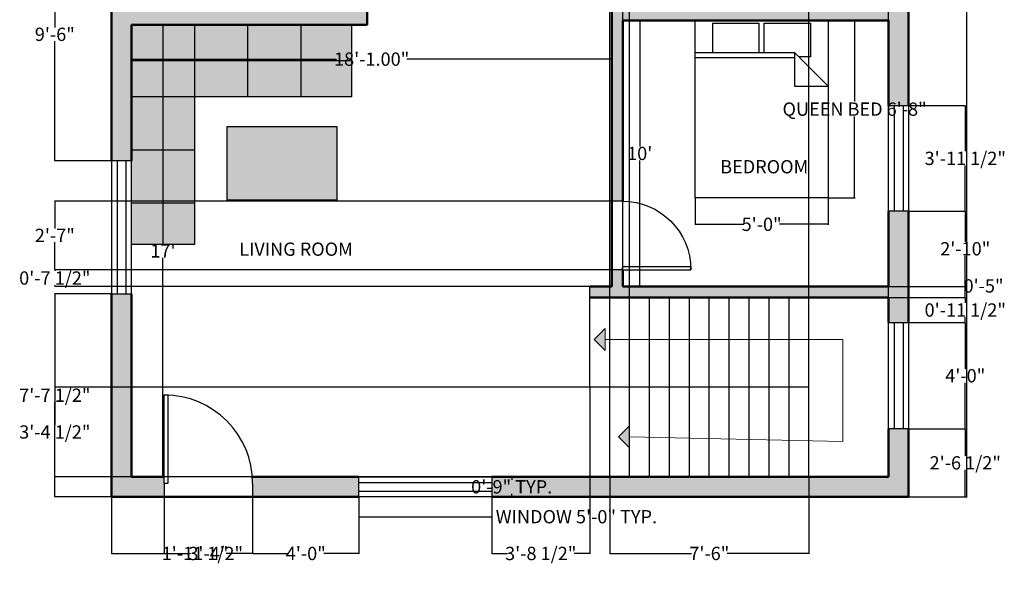
# Model space of a CAD drawing. Units: inches. Extents: x -19 to 426, y -15 to 535.
# Tile 1 of 4: x -19 to 426, y -15 to 235. Entities that reach past the tile are written whole.
import ezdxf

# ---------------------------------------------------------------- set-up
doc = ezdxf.new("R2010")
doc.units = ezdxf.units.IN
doc.header["$MEASUREMENT"] = 0
for name, color, linetype, lineweight in [('A-ANNO-DIMS', 3, 'Continuous', 18), ('A-ANNO-PATT', 18, 'Continuous', 13), ('A-ANNO-SYMB', 7, 'Continuous', 18), ('A-AREA-IDEN', 7, 'Continuous', 25), ('A-DOOR', 4, 'Continuous', 25), ('A-FLOR-STRS', 7, 'Continuous', 25), ('A-FURN', 40, 'Continuous', 25), ('A-FURN-PATT', 9, 'Continuous', 13), ('A-GLAZ', 40, 'Continuous', 25), ('A-WALL', 7, 'Continuous', 50), ('A-WALL-PATT', 5, 'Continuous', 13)]:
    doc.layers.add(name, color=color, linetype=linetype, lineweight=lineweight)
doc.styles.get("Standard").update_dxf_attribs({"font": 'arial.ttf'})
doc.dimstyles.get("Standard").update_dxf_attribs({"dimtxt": 6, "dimasz": 0.18, "dimexe": 0.18, "dimexo": 0.0625, "dimgap": 0.09, "dimtad": 0, "dimtih": 1, "dimtoh": 1, "dimzin": 0, "dimdsep": 46, "dimlunit": 3, "dimtxsty": 'Standard', "dimcen": 0.09, "dimadec": 0, "dimazin": 0, "dimtfac": 1, "dimtofl": 0, "dimtmove": 0, "dimatfit": 3, "dimfxl": 1, "dimtolj": 1, "dimtzin": 0, "dimarcsym": 0})

# ---------------------------------------------------------------- blocks, each defined once
blk = doc.blocks.new('*D1')
at = {"layer": 'A-ANNO-DIMS', "color": 0, "lineweight": -2, "transparency": 16777216}
for p, q in [((253.49, 235.01), (261.17, 235.01)), ((260.99, 234.83), (260.99, 178.16)), ((260.99, 115.19), (260.99, 171.85)), ((253.49, 115.01), (261.17, 115.01))]:
    blk.add_line(p, q, dxfattribs=at)
at = {"layer": 'A-ANNO-DIMS', "color": 0, "transparency": 16777216}
for points in [[(260.96, 234.83), (261.02, 234.83), (260.99, 235.01)], [(260.96, 115.19), (261.02, 115.19), (260.99, 115.01)]]:
    blk.add_solid(points, dxfattribs=at)
at = {"layer": 'Defpoints', "color": 0, "transparency": 16777216}
for p in [(253.43, 235.01), (260.99, 235.01), (253.43, 115.01)]:
    blk.add_point(p, dxfattribs=at)
at = {"layer": 'A-ANNO-DIMS', "color": 0, "transparency": 16777216, "insert": (260.99, 175.01), "char_height": 6, "attachment_point": 5}
blk.add_mtext("\\A1;10'", dxfattribs=at)
blk = doc.blocks.new('Bed - Queen')
for p, q in [((0, -80.00003), (0, 0)), ((0, 0), (59.99999, 0)), ((59.99999, 0), (59.99999, -80.00003)), ((7.99999, -1.2), (28.79998, -1.2)), ((7.99999, -14.4), (7.99999, -1.2)), ((28.79998, -1.2), (28.79998, -14.4)), ((31.19999, -1.2), (51.99999, -1.2)), ((31.19999, -14.4), (31.19999, -1.2)), ((51.99999, -1.2), (51.99999, -16.4)), ((0, -14.4), (44.8, -14.4)), ((44.8, -16.8), (0, -16.8)), ((59.99999, -29.6), (44.8, -14.4)), ((44.8, -14.4), (44.8, -29.6)), ((51.99999, -16.4), (46.79936, -16.4)), ((44.8, -29.6), (59.99999, -29.6)), ((59.99999, -80.00003), (0, -80.00003))]:
    blk.add_line(p, q)
blk = doc.blocks.new('*U9')
for p, q in [((0, 0), (0, -6)), ((40, 0), (40, -6))]:
    blk.add_line(p, q)
blk.add_lwpolyline([(0, 0), (0, 40), (1.75, 40), (1.75, 0)], close=True)
blk.add_arc((0, 0), 40, 0, 90)
blk = doc.blocks.new('*D16')
at = {"layer": 'A-ANNO-DIMS', "color": 0, "lineweight": -2, "transparency": 16777216}
for p, q in [((31.43, 232.94), (31.43, 217.39)), ((248.43, 232.94), (248.43, 217.39)), ((31.61, 217.57), (123.99, 217.57)), ((248.25, 217.57), (155.87, 217.57))]:
    blk.add_line(p, q, dxfattribs=at)
at = {"layer": 'A-ANNO-DIMS', "color": 0, "transparency": 16777216}
for points in [[(31.61, 217.6), (31.61, 217.54), (31.43, 217.57)], [(248.25, 217.6), (248.25, 217.54), (248.43, 217.57)]]:
    blk.add_solid(points, dxfattribs=at)
at = {"layer": 'Defpoints', "color": 0, "transparency": 16777216}
for p in [(31.43, 233.01), (248.43, 233.01), (248.43, 217.57)]:
    blk.add_point(p, dxfattribs=at)
at = {"layer": 'A-ANNO-DIMS', "color": 0, "transparency": 16777216, "insert": (139.93, 217.57), "char_height": 6, "attachment_point": 5}
blk.add_mtext('\\A1;18\'-1.00"', dxfattribs=at)
blk = doc.blocks.new('*D17')
at = {"layer": 'A-ANNO-DIMS', "color": 0, "lineweight": -2, "transparency": 16777216}
for p, q in [((31.49, 233.01), (45.84, 233.01)), ((45.66, 232.83), (45.66, 134.11)), ((45.66, 29.19), (45.66, 127.9)), ((31.49, 29.01), (45.84, 29.01))]:
    blk.add_line(p, q, dxfattribs=at)
at = {"layer": 'A-ANNO-DIMS', "color": 0, "transparency": 16777216}
for points in [[(45.63, 232.83), (45.69, 232.83), (45.66, 233.01)], [(45.63, 29.19), (45.69, 29.19), (45.66, 29.01)]]:
    blk.add_solid(points, dxfattribs=at)
at = {"layer": 'Defpoints', "color": 0, "transparency": 16777216}
for p in [(31.43, 233.01), (45.66, 233.01), (31.43, 29.01)]:
    blk.add_point(p, dxfattribs=at)
at = {"layer": 'A-ANNO-DIMS', "color": 0, "transparency": 16777216, "insert": (45.66, 131.01), "char_height": 6, "attachment_point": 5}
blk.add_mtext("\\A1;17'", dxfattribs=at)
blk = doc.blocks.new('*D19')
at = {"layer": 'A-ANNO-DIMS', "color": 0, "lineweight": -2, "transparency": 16777216}
for p, q in [((382.49, 500.01), (408.92, 500.01)), ((408.74, 499.83), (408.74, 263.16)), ((408.74, 20.19), (408.74, 256.85)), ((382.49, 20.01), (408.92, 20.01))]:
    blk.add_line(p, q, dxfattribs=at)
at = {"layer": 'A-ANNO-DIMS', "color": 0, "transparency": 16777216}
for points in [[(408.71, 499.83), (408.77, 499.83), (408.74, 500.01)], [(408.71, 20.19), (408.77, 20.19), (408.74, 20.01)]]:
    blk.add_solid(points, dxfattribs=at)
at = {"layer": 'Defpoints', "color": 0, "transparency": 16777216}
for p in [(382.43, 500.01), (382.43, 20.01), (408.74, 20.01)]:
    blk.add_point(p, dxfattribs=at)
at = {"layer": 'A-ANNO-DIMS', "color": 0, "transparency": 16777216, "insert": (408.74, 260.01), "char_height": 6, "attachment_point": 5}
blk.add_mtext("\\A1;40'", dxfattribs=at)
blk = doc.blocks.new('WIN-60IN')
for p, q in [((0, 6.5), (60, 6.5)), ((0, 2.5), (60, 2.5))]:
    blk.add_line(p, q)
blk.add_lwpolyline([(0, 9), (60, 9), (60, 0), (0, 0)], close=True)
blk = doc.blocks.new('*D22')
at = {"layer": 'A-ANNO-DIMS', "color": 0, "lineweight": -2, "transparency": 16777216}
for p, q in [((134.17, 19.94), (134.17, 10.83)), ((194.17, 19.94), (194.17, 10.83)), ((134.35, 11.01), (193.99, 11.01)), ((194.17, 11.01), (194.35, 11.01))]:
    blk.add_line(p, q, dxfattribs=at)
at = {"layer": 'A-ANNO-DIMS', "color": 0, "transparency": 16777216}
for points in [[(134.35, 11.04), (134.35, 10.98), (134.17, 11.01)], [(193.99, 11.04), (193.99, 10.98), (194.17, 11.01)]]:
    blk.add_solid(points, dxfattribs=at)
at = {"layer": 'Defpoints', "color": 0, "transparency": 16777216}
for p in [(134.17, 20.01), (194.17, 20.01), (194.17, 11.01)]:
    blk.add_point(p, dxfattribs=at)
at = {"layer": 'A-ANNO-DIMS', "color": 0, "transparency": 16777216, "insert": (232.4, 11.01), "char_height": 6, "attachment_point": 5}
blk.add_mtext('\\A1;WINDOW 5\'-0" TYP.', dxfattribs=at)
blk = doc.blocks.new('*D23')
at = {"layer": 'A-ANNO-DIMS', "color": 0, "lineweight": -2, "transparency": 16777216}
for p, q in [((194.23, 29.01), (203.35, 29.01)), ((203.17, 28.83), (203.17, 27.66)), ((194.23, 20.01), (203.35, 20.01)), ((203.17, 20.19), (203.17, 21.35))]:
    blk.add_line(p, q, dxfattribs=at)
at = {"layer": 'A-ANNO-DIMS', "color": 0, "transparency": 16777216}
for points in [[(203.14, 28.83), (203.2, 28.83), (203.17, 29.01)], [(203.14, 20.19), (203.2, 20.19), (203.17, 20.01)]]:
    blk.add_solid(points, dxfattribs=at)
at = {"layer": 'Defpoints', "color": 0, "transparency": 16777216}
for p in [(194.17, 29.01), (203.17, 29.01), (194.17, 20.01)]:
    blk.add_point(p, dxfattribs=at)
at = {"layer": 'A-ANNO-DIMS', "color": 0, "transparency": 16777216, "insert": (203.17, 24.51), "char_height": 6, "attachment_point": 5}
blk.add_mtext('\\A1;0\'-9" TYP.', dxfattribs=at)
blk = doc.blocks.new('*D26')
at = {"layer": 'A-ANNO-DIMS', "color": 0, "lineweight": -2, "transparency": 16777216}
for p, q in [((346.12, 235.01), (358.24, 235.01)), ((358.06, 234.83), (358.06, 198.38)), ((358.06, 155.19), (358.06, 191.63)), ((346.12, 155.01), (358.24, 155.01))]:
    blk.add_line(p, q, dxfattribs=at)
at = {"layer": 'A-ANNO-DIMS', "color": 0, "transparency": 16777216}
for points in [[(358.03, 234.83), (358.09, 234.83), (358.06, 235.01)], [(358.03, 155.19), (358.09, 155.19), (358.06, 155.01)]]:
    blk.add_solid(points, dxfattribs=at)
at = {"layer": 'Defpoints', "color": 0, "transparency": 16777216}
for p in [(346.06, 235.01), (358.06, 235.01), (346.06, 155.01)]:
    blk.add_point(p, dxfattribs=at)
at = {"layer": 'A-ANNO-DIMS', "color": 0, "transparency": 16777216, "insert": (358.06, 195.01), "char_height": 6, "attachment_point": 5}
blk.add_mtext('\\A1;QUEEN BED 6\'-8"', dxfattribs=at)
blk = doc.blocks.new('*D27')
at = {"layer": 'A-ANNO-DIMS', "color": 0, "lineweight": -2, "transparency": 16777216}
for p, q in [((286.06, 154.94), (286.06, 142.83)), ((346.06, 154.94), (346.06, 142.83)), ((286.24, 143.01), (307.99, 143.01)), ((345.88, 143.01), (324.12, 143.01))]:
    blk.add_line(p, q, dxfattribs=at)
at = {"layer": 'A-ANNO-DIMS', "color": 0, "transparency": 16777216}
for points in [[(286.24, 143.04), (286.24, 142.98), (286.06, 143.01)], [(345.88, 143.04), (345.88, 142.98), (346.06, 143.01)]]:
    blk.add_solid(points, dxfattribs=at)
at = {"layer": 'Defpoints', "color": 0, "transparency": 16777216}
for p in [(286.06, 155.01), (346.06, 155.01), (346.06, 143.01)]:
    blk.add_point(p, dxfattribs=at)
at = {"layer": 'A-ANNO-DIMS', "color": 0, "transparency": 16777216, "insert": (316.06, 143.01), "char_height": 6, "attachment_point": 5}
blk.add_mtext('\\A1;5\'-0"', dxfattribs=at)
blk = doc.blocks.new('*D32')
at = {"layer": 'A-ANNO-DIMS', "color": 0, "lineweight": -2, "transparency": 16777216}
for p, q in [((253.43, 115.07), (253.43, 525.79)), ((253.61, 525.61), (303.32, 525.61)), ((373.25, 525.61), (323.55, 525.61)), ((373.43, 115.07), (373.43, 525.79))]:
    blk.add_line(p, q, dxfattribs=at)
at = {"layer": 'A-ANNO-DIMS', "color": 0, "transparency": 16777216}
for points in [[(253.61, 525.64), (253.61, 525.58), (253.43, 525.61)], [(373.25, 525.64), (373.25, 525.58), (373.43, 525.61)]]:
    blk.add_solid(points, dxfattribs=at)
at = {"layer": 'Defpoints', "color": 0, "transparency": 16777216}
for p in [(373.43, 525.61), (253.43, 115.01), (373.43, 115.01)]:
    blk.add_point(p, dxfattribs=at)
at = {"layer": 'A-ANNO-DIMS', "color": 0, "transparency": 16777216, "insert": (313.43, 525.61), "char_height": 6, "attachment_point": 5}
blk.add_mtext('\\A1;10\'-0"', dxfattribs=at)
blk = doc.blocks.new('*D33')
at = {"layer": 'A-ANNO-DIMS', "color": 0, "lineweight": -2, "transparency": 16777216}
for p, q in [((238.43, 69.44), (238.43, -5.77)), ((194.17, 19.94), (194.17, -5.77)), ((194.35, -5.59), (201.25, -5.59)), ((238.25, -5.59), (231.35, -5.59))]:
    blk.add_line(p, q, dxfattribs=at)
at = {"layer": 'A-ANNO-DIMS', "color": 0, "transparency": 16777216}
for points in [[(194.35, -5.56), (194.35, -5.62), (194.17, -5.59)], [(238.25, -5.56), (238.25, -5.62), (238.43, -5.59)]]:
    blk.add_solid(points, dxfattribs=at)
at = {"layer": 'Defpoints', "color": 0, "transparency": 16777216}
for p in [(238.43, 69.51), (194.17, 20.01), (238.43, -5.59)]:
    blk.add_point(p, dxfattribs=at)
at = {"layer": 'A-ANNO-DIMS', "color": 0, "transparency": 16777216, "insert": (216.3, -5.59), "char_height": 6, "attachment_point": 5}
blk.add_mtext('\\A1;3\'-8 1/2"', dxfattribs=at)
blk = doc.blocks.new('*D34')
at = {"layer": 'A-ANNO-DIMS', "color": 0, "lineweight": -2, "transparency": 16777216}
for p, q in [((22.43, 19.94), (22.43, -5.77)), ((46.18, 19.94), (46.18, -5.77)), ((22.61, -5.59), (46, -5.59)), ((46.18, -5.59), (46.36, -5.59))]:
    blk.add_line(p, q, dxfattribs=at)
at = {"layer": 'A-ANNO-DIMS', "color": 0, "transparency": 16777216}
for points in [[(22.61, -5.56), (22.61, -5.62), (22.43, -5.59)], [(46, -5.56), (46, -5.62), (46.18, -5.59)]]:
    blk.add_solid(points, dxfattribs=at)
at = {"layer": 'Defpoints', "color": 0, "transparency": 16777216}
for p in [(22.43, 20.01), (46.18, 20.01), (46.18, -5.59)]:
    blk.add_point(p, dxfattribs=at)
at = {"layer": 'A-ANNO-DIMS', "color": 0, "transparency": 16777216, "insert": (63.47, -5.59), "char_height": 6, "attachment_point": 5}
blk.add_mtext('\\A1;1\'-11 1/2"', dxfattribs=at)
blk = doc.blocks.new('*D35')
at = {"layer": 'A-ANNO-DIMS', "color": 0, "lineweight": -2, "transparency": 16777216}
for p, q in [((46.18, 19.94), (46.18, -5.77)), ((86.18, 19.94), (86.18, -5.77)), ((46.36, -5.59), (58.12, -5.59)), ((86, -5.59), (74.24, -5.59))]:
    blk.add_line(p, q, dxfattribs=at)
at = {"layer": 'A-ANNO-DIMS', "color": 0, "transparency": 16777216}
for points in [[(46.36, -5.56), (46.36, -5.62), (46.18, -5.59)], [(86, -5.56), (86, -5.62), (86.18, -5.59)]]:
    blk.add_solid(points, dxfattribs=at)
at = {"layer": 'Defpoints', "color": 0, "transparency": 16777216}
for p in [(46.18, 20.01), (86.18, 20.01), (86.18, -5.59)]:
    blk.add_point(p, dxfattribs=at)
at = {"layer": 'A-ANNO-DIMS', "color": 0, "transparency": 16777216, "insert": (66.18, -5.59), "char_height": 6, "attachment_point": 5}
blk.add_mtext('\\A1;3\'-4"', dxfattribs=at)
blk = doc.blocks.new('*D36')
at = {"layer": 'A-ANNO-DIMS', "color": 0, "lineweight": -2, "transparency": 16777216}
for p, q in [((86.18, 19.94), (86.18, -5.77)), ((134.17, 19.94), (134.17, -5.77)), ((86.36, -5.59), (101.99, -5.59)), ((133.99, -5.59), (118.36, -5.59))]:
    blk.add_line(p, q, dxfattribs=at)
at = {"layer": 'A-ANNO-DIMS', "color": 0, "transparency": 16777216}
for points in [[(86.36, -5.56), (86.36, -5.62), (86.18, -5.59)], [(133.99, -5.56), (133.99, -5.62), (134.17, -5.59)]]:
    blk.add_solid(points, dxfattribs=at)
at = {"layer": 'Defpoints', "color": 0, "transparency": 16777216}
for p in [(86.18, 20.01), (134.17, 20.01), (134.17, -5.59)]:
    blk.add_point(p, dxfattribs=at)
at = {"layer": 'A-ANNO-DIMS', "color": 0, "transparency": 16777216, "insert": (110.18, -5.59), "char_height": 6, "attachment_point": 5}
blk.add_mtext('\\A1;4\'-0"', dxfattribs=at)
blk = doc.blocks.new('*D38')
at = {"layer": 'A-ANNO-DIMS', "color": 0, "lineweight": -2, "transparency": 16777216}
for p, q in [((22.37, 111.69), (-3.35, 111.69)), ((-3.17, 111.51), (-3.17, 69.04)), ((-3.17, 20.19), (-3.17, 62.66)), ((22.37, 20.01), (-3.35, 20.01))]:
    blk.add_line(p, q, dxfattribs=at)
at = {"layer": 'A-ANNO-DIMS', "color": 0, "transparency": 16777216}
for points in [[(-3.2, 111.51), (-3.14, 111.51), (-3.17, 111.69)], [(-3.2, 20.19), (-3.14, 20.19), (-3.17, 20.01)]]:
    blk.add_solid(points, dxfattribs=at)
at = {"layer": 'Defpoints', "color": 0, "transparency": 16777216}
for p in [(-3.17, 111.69), (22.43, 111.69), (22.43, 20.01)]:
    blk.add_point(p, dxfattribs=at)
at = {"layer": 'A-ANNO-DIMS', "color": 0, "transparency": 16777216, "insert": (-3.17, 65.85), "char_height": 6, "attachment_point": 5}
blk.add_mtext('\\A1;7\'-7 1/2"', dxfattribs=at)
blk = doc.blocks.new('*D39')
at = {"layer": 'A-ANNO-DIMS', "color": 0, "lineweight": -2, "transparency": 16777216}
for p, q in [((22.37, 285.87), (-3.35, 285.87)), ((-3.17, 285.69), (-3.17, 231.93)), ((-3.17, 171.87), (-3.17, 225.63)), ((22.37, 171.69), (-3.35, 171.69))]:
    blk.add_line(p, q, dxfattribs=at)
at = {"layer": 'A-ANNO-DIMS', "color": 0, "transparency": 16777216}
for points in [[(-3.2, 285.69), (-3.14, 285.69), (-3.17, 285.87)], [(-3.2, 171.87), (-3.14, 171.87), (-3.17, 171.69)]]:
    blk.add_solid(points, dxfattribs=at)
at = {"layer": 'Defpoints', "color": 0, "transparency": 16777216}
for p in [(-3.17, 285.87), (22.43, 285.87), (22.43, 171.69)]:
    blk.add_point(p, dxfattribs=at)
at = {"layer": 'A-ANNO-DIMS', "color": 0, "transparency": 16777216, "insert": (-3.17, 228.78), "char_height": 6, "attachment_point": 5}
blk.add_mtext('\\A1;9\'-6"', dxfattribs=at)
blk = doc.blocks.new('*D43')
at = {"layer": 'A-ANNO-DIMS', "color": 0, "lineweight": -2, "transparency": 16777216}
for p, q in [((382.49, 50.63), (408.21, 50.63)), ((408.03, 50.45), (408.03, 38.51)), ((408.03, 20.19), (408.03, 32.13)), ((382.49, 20.01), (408.21, 20.01))]:
    blk.add_line(p, q, dxfattribs=at)
at = {"layer": 'A-ANNO-DIMS', "color": 0, "transparency": 16777216}
for points in [[(408, 50.45), (408.06, 50.45), (408.03, 50.63)], [(408, 20.19), (408.06, 20.19), (408.03, 20.01)]]:
    blk.add_solid(points, dxfattribs=at)
at = {"layer": 'Defpoints', "color": 0, "transparency": 16777216}
for p in [(382.43, 50.63), (408.03, 50.63), (382.43, 20.01)]:
    blk.add_point(p, dxfattribs=at)
at = {"layer": 'A-ANNO-DIMS', "color": 0, "transparency": 16777216, "insert": (408.03, 35.32), "char_height": 6, "attachment_point": 5}
blk.add_mtext('\\A1;2\'-6 1/2"', dxfattribs=at)
blk = doc.blocks.new('*D44')
at = {"layer": 'A-ANNO-DIMS', "color": 0, "lineweight": -2, "transparency": 16777216}
for p, q in [((382.49, 98.63), (408.21, 98.63)), ((408.03, 98.45), (408.03, 77.79)), ((408.03, 50.81), (408.03, 71.48)), ((382.49, 50.63), (408.21, 50.63))]:
    blk.add_line(p, q, dxfattribs=at)
at = {"layer": 'A-ANNO-DIMS', "color": 0, "transparency": 16777216}
for points in [[(408, 98.45), (408.06, 98.45), (408.03, 98.63)], [(408, 50.81), (408.06, 50.81), (408.03, 50.63)]]:
    blk.add_solid(points, dxfattribs=at)
at = {"layer": 'Defpoints', "color": 0, "transparency": 16777216}
for p in [(382.43, 98.63), (408.03, 98.63), (382.43, 50.63)]:
    blk.add_point(p, dxfattribs=at)
at = {"layer": 'A-ANNO-DIMS', "color": 0, "transparency": 16777216, "insert": (408.03, 74.63), "char_height": 6, "attachment_point": 5}
blk.add_mtext('\\A1;4\'-0"', dxfattribs=at)
blk = doc.blocks.new('*D45')
at = {"layer": 'A-ANNO-DIMS', "color": 0, "lineweight": -2, "transparency": 16777216}
for p, q in [((373.49, 110.01), (408.21, 110.01)), ((408.03, 109.83), (408.03, 107.51)), ((382.49, 98.63), (408.21, 98.63)), ((408.03, 98.81), (408.03, 101.13))]:
    blk.add_line(p, q, dxfattribs=at)
at = {"layer": 'A-ANNO-DIMS', "color": 0, "transparency": 16777216}
for points in [[(408, 109.83), (408.06, 109.83), (408.03, 110.01)], [(408, 98.81), (408.06, 98.81), (408.03, 98.63)]]:
    blk.add_solid(points, dxfattribs=at)
at = {"layer": 'Defpoints', "color": 0, "transparency": 16777216}
for p in [(373.43, 110.01), (408.03, 110.01), (382.43, 98.63)]:
    blk.add_point(p, dxfattribs=at)
at = {"layer": 'A-ANNO-DIMS', "color": 0, "transparency": 16777216, "insert": (408.03, 104.32), "char_height": 6, "attachment_point": 5}
blk.add_mtext('\\A1;0\'-11 1/2"', dxfattribs=at)
blk = doc.blocks.new('*D46')
at = {"layer": 'A-ANNO-DIMS', "color": 0, "lineweight": -2, "transparency": 16777216}
for p, q in [((382.49, 148.92), (408.21, 148.92)), ((408.03, 148.74), (408.03, 135.12)), ((408.03, 115.19), (408.03, 128.81)), ((373.49, 115.01), (408.21, 115.01))]:
    blk.add_line(p, q, dxfattribs=at)
at = {"layer": 'A-ANNO-DIMS', "color": 0, "transparency": 16777216}
for points in [[(408, 148.74), (408.06, 148.74), (408.03, 148.92)], [(408, 115.19), (408.06, 115.19), (408.03, 115.01)]]:
    blk.add_solid(points, dxfattribs=at)
at = {"layer": 'Defpoints', "color": 0, "transparency": 16777216}
for p in [(382.43, 148.92), (408.03, 148.92), (373.43, 115.01)]:
    blk.add_point(p, dxfattribs=at)
at = {"layer": 'A-ANNO-DIMS', "color": 0, "transparency": 16777216, "insert": (408.03, 131.96), "char_height": 6, "attachment_point": 5}
blk.add_mtext('\\A1;2\'-10"', dxfattribs=at)
blk = doc.blocks.new('*D47')
at = {"layer": 'A-ANNO-DIMS', "color": 0, "lineweight": -2, "transparency": 16777216}
for p, q in [((382.49, 196.66), (408.21, 196.66)), ((408.03, 196.48), (408.03, 175.99)), ((408.03, 149.1), (408.03, 169.6)), ((382.49, 148.92), (408.21, 148.92))]:
    blk.add_line(p, q, dxfattribs=at)
at = {"layer": 'A-ANNO-DIMS', "color": 0, "transparency": 16777216}
for points in [[(408, 196.48), (408.06, 196.48), (408.03, 196.66)], [(408, 149.1), (408.06, 149.1), (408.03, 148.92)]]:
    blk.add_solid(points, dxfattribs=at)
at = {"layer": 'Defpoints', "color": 0, "transparency": 16777216}
for p in [(382.43, 196.66), (408.03, 196.66), (382.43, 148.92)]:
    blk.add_point(p, dxfattribs=at)
at = {"layer": 'A-ANNO-DIMS', "color": 0, "transparency": 16777216, "insert": (408.03, 172.79), "char_height": 6, "attachment_point": 5}
blk.add_mtext('\\A1;3\'-11 1/2"', dxfattribs=at)
blk = doc.blocks.new('*D57')
at = {"layer": 'A-ANNO-DIMS', "color": 0, "lineweight": -2, "transparency": 16777216}
for p, q in [((248.37, 122.52), (-3.35, 122.52)), ((-3.17, 122.34), (-3.17, 121.95)), ((248.37, 115.01), (-3.35, 115.01)), ((-3.17, 115.19), (-3.17, 115.57))]:
    blk.add_line(p, q, dxfattribs=at)
at = {"layer": 'A-ANNO-DIMS', "color": 0, "transparency": 16777216}
for points in [[(-3.2, 122.34), (-3.14, 122.34), (-3.17, 122.52)], [(-3.2, 115.19), (-3.14, 115.19), (-3.17, 115.01)]]:
    blk.add_solid(points, dxfattribs=at)
at = {"layer": 'Defpoints', "color": 0, "transparency": 16777216}
for p in [(-3.17, 122.52), (248.43, 122.52), (248.43, 115.01)]:
    blk.add_point(p, dxfattribs=at)
at = {"layer": 'A-ANNO-DIMS', "color": 0, "transparency": 16777216, "insert": (-3.17, 118.76), "char_height": 6, "attachment_point": 5}
blk.add_mtext('\\A1;0\'-7 1/2"', dxfattribs=at)
blk = doc.blocks.new('*D58')
at = {"layer": 'A-ANNO-DIMS', "color": 0, "lineweight": -2, "transparency": 16777216}
for p, q in [((248.37, 153.52), (-3.35, 153.52)), ((-3.17, 153.34), (-3.17, 141.12)), ((-3.17, 122.7), (-3.17, 134.91)), ((248.37, 122.52), (-3.35, 122.52))]:
    blk.add_line(p, q, dxfattribs=at)
at = {"layer": 'A-ANNO-DIMS', "color": 0, "transparency": 16777216}
for points in [[(-3.2, 153.34), (-3.14, 153.34), (-3.17, 153.52)], [(-3.2, 122.7), (-3.14, 122.7), (-3.17, 122.52)]]:
    blk.add_solid(points, dxfattribs=at)
at = {"layer": 'Defpoints', "color": 0, "transparency": 16777216}
for p in [(-3.17, 153.52), (248.43, 153.52), (248.43, 122.52)]:
    blk.add_point(p, dxfattribs=at)
at = {"layer": 'A-ANNO-DIMS', "color": 0, "transparency": 16777216, "insert": (-3.17, 138.02), "char_height": 6, "attachment_point": 5}
blk.add_mtext('\\A1;2\'-7"', dxfattribs=at)
blk = doc.blocks.new('*D60')
at = {"layer": 'A-ANNO-DIMS', "color": 0, "lineweight": -2, "transparency": 16777216}
for p, q in [((373.49, 115.01), (408.21, 115.01)), ((408.03, 115.01), (408.03, 115.19)), ((408.03, 115.19), (408.21, 115.19)), ((408.03, 110.19), (408.03, 114.83)), ((373.49, 110.01), (408.21, 110.01))]:
    blk.add_line(p, q, dxfattribs=at)
at = {"layer": 'A-ANNO-DIMS', "color": 0, "transparency": 16777216}
for points in [[(408, 114.83), (408.06, 114.83), (408.03, 115.01)], [(408, 110.19), (408.06, 110.19), (408.03, 110.01)]]:
    blk.add_solid(points, dxfattribs=at)
at = {"layer": 'Defpoints', "color": 0, "transparency": 16777216}
for p in [(373.43, 115.01), (408.03, 115.01), (373.43, 110.01)]:
    blk.add_point(p, dxfattribs=at)
at = {"layer": 'A-ANNO-DIMS', "color": 0, "transparency": 16777216, "insert": (416.28, 115.19), "char_height": 6, "attachment_point": 5}
blk.add_mtext('\\A1;0\'-5"', dxfattribs=at)
blk = doc.blocks.new('*D61')
at = {"layer": 'A-ANNO-DIMS', "color": 0, "lineweight": -2, "transparency": 16777216}
for p, q in [((247.43, 29.07), (247.43, 525.79)), ((247.61, 525.61), (256.25, 525.61)), ((256.43, 29.07), (256.43, 525.79)), ((256.43, 525.61), (256.61, 525.61))]:
    blk.add_line(p, q, dxfattribs=at)
at = {"layer": 'A-ANNO-DIMS', "color": 0, "transparency": 16777216}
for points in [[(247.61, 525.64), (247.61, 525.58), (247.43, 525.61)], [(256.25, 525.64), (256.25, 525.58), (256.43, 525.61)]]:
    blk.add_solid(points, dxfattribs=at)
at = {"layer": 'Defpoints', "color": 0, "transparency": 16777216}
for p in [(256.43, 525.61), (247.43, 29.01), (256.43, 29.01)]:
    blk.add_point(p, dxfattribs=at)
at = {"layer": 'A-ANNO-DIMS', "color": 0, "transparency": 16777216, "insert": (264.68, 525.61), "char_height": 6, "attachment_point": 5}
blk.add_mtext('\\A1;0\'-9"', dxfattribs=at)
blk = doc.blocks.new('*D62')
at = {"layer": 'A-ANNO-DIMS', "color": 0, "lineweight": -2, "transparency": 16777216}
for p, q in [((337.43, 29.07), (337.43, 525.79)), ((337.61, 525.61), (347.37, 525.61)), ((373.25, 525.61), (363.5, 525.61)), ((373.43, 29.07), (373.43, 525.79))]:
    blk.add_line(p, q, dxfattribs=at)
at = {"layer": 'A-ANNO-DIMS', "color": 0, "transparency": 16777216}
for points in [[(337.61, 525.64), (337.61, 525.58), (337.43, 525.61)], [(373.25, 525.64), (373.25, 525.58), (373.43, 525.61)]]:
    blk.add_solid(points, dxfattribs=at)
at = {"layer": 'Defpoints', "color": 0, "transparency": 16777216}
for p in [(373.43, 525.61), (337.43, 29.01), (373.43, 29.01)]:
    blk.add_point(p, dxfattribs=at)
at = {"layer": 'A-ANNO-DIMS', "color": 0, "transparency": 16777216, "insert": (355.43, 525.61), "char_height": 6, "attachment_point": 5}
blk.add_mtext('\\A1;3\'-0"', dxfattribs=at)
blk = doc.blocks.new('*D63')
at = {"layer": 'A-ANNO-DIMS', "color": 0, "lineweight": -2, "transparency": 16777216}
for p, q in [((238.37, 69.51), (-3.35, 69.51)), ((-3.17, 69.33), (-3.17, 52.45)), ((-3.17, 29.19), (-3.17, 46.06)), ((247.37, 29.01), (-3.35, 29.01))]:
    blk.add_line(p, q, dxfattribs=at)
at = {"layer": 'A-ANNO-DIMS', "color": 0, "transparency": 16777216}
for points in [[(-3.2, 69.33), (-3.14, 69.33), (-3.17, 69.51)], [(-3.2, 29.19), (-3.14, 29.19), (-3.17, 29.01)]]:
    blk.add_solid(points, dxfattribs=at)
at = {"layer": 'Defpoints', "color": 0, "transparency": 16777216}
for p in [(-3.17, 69.51), (238.43, 69.51), (247.43, 29.01)]:
    blk.add_point(p, dxfattribs=at)
at = {"layer": 'A-ANNO-DIMS', "color": 0, "transparency": 16777216, "insert": (-3.17, 49.26), "char_height": 6, "attachment_point": 5}
blk.add_mtext('\\A1;3\'-4 1/2"', dxfattribs=at)
blk = doc.blocks.new('*D64')
at = {"layer": 'A-ANNO-DIMS', "color": 0, "lineweight": -2, "transparency": 16777216}
for p, q in [((247.43, 28.94), (247.43, -5.77)), ((337.43, 28.94), (337.43, -5.77)), ((247.61, -5.59), (284.39, -5.59)), ((337.25, -5.59), (300.47, -5.59))]:
    blk.add_line(p, q, dxfattribs=at)
at = {"layer": 'A-ANNO-DIMS', "color": 0, "transparency": 16777216}
for points in [[(247.61, -5.56), (247.61, -5.62), (247.43, -5.59)], [(337.25, -5.56), (337.25, -5.62), (337.43, -5.59)]]:
    blk.add_solid(points, dxfattribs=at)
at = {"layer": 'Defpoints', "color": 0, "transparency": 16777216}
for p in [(247.43, 29.01), (337.43, 29.01), (337.43, -5.59)]:
    blk.add_point(p, dxfattribs=at)
at = {"layer": 'A-ANNO-DIMS', "color": 0, "transparency": 16777216, "insert": (292.43, -5.59), "char_height": 6, "attachment_point": 5}
blk.add_mtext('\\A1;7\'-6"', dxfattribs=at)

msp = doc.modelspace()

# ---------------------------------------------------------------- hatches: boundary and pattern name
at = {"layer": 'A-ANNO-PATT'}
h = msp.add_hatch(color=256, dxfattribs=at)
h.dxf.hatch_style = 1
h.paths.add_polyline_path([(256.432, 52.06), (251.432, 47.06), (256.432, 42.06), (256.432, 47.06)])
h.paths.add_polyline_path([(245.426, 95.99), (240.426, 90.99), (245.426, 85.99), (245.426, 90.99)])
at = {"layer": 'A-FURN-PATT'}
h = msp.add_hatch(color=256, dxfattribs=at)
h.dxf.hatch_style = 1
h.paths.add_polyline_path([(45.659, 152.508), (31.432, 152.508), (31.432, 133.911), (45.659, 133.911)])
h.paths.add_polyline_path([(45.659, 176.508), (31.432, 176.508), (31.432, 152.508), (45.659, 152.508)])
h.paths.add_polyline_path([(45.659, 200.508), (31.432, 200.508), (31.432, 176.508), (45.659, 176.508)])
h.paths.add_polyline_path([(45.659, 216.757), (31.432, 216.757), (31.432, 200.508), (45.659, 200.508)])
h.paths.add_polyline_path([(45.659, 233.007), (31.432, 233.007), (31.432, 216.757), (45.659, 216.757)])
h.paths.add_polyline_path([(59.885, 233.007), (45.659, 233.007), (45.659, 216.757), (59.885, 216.757)])
h.paths.add_polyline_path([(83.885, 233.007), (59.885, 233.007), (59.885, 216.757), (83.885, 216.757)])
h.paths.add_polyline_path([(107.885, 233.007), (83.885, 233.007), (83.885, 216.757), (107.885, 216.757)])
h.paths.add_polyline_path([(130.834, 233.007), (107.885, 233.007), (107.885, 216.757), (130.834, 216.757)])
h.paths.add_polyline_path([(121.67, 218.649), (157.675, 218.649), (157.675, 231.013), (121.67, 231.013)], flags=9)
h = msp.add_hatch(color=256, dxfattribs=at)
h.dxf.hatch_style = 1
h.paths.add_polyline_path([(130.834, 233.007), (107.885, 233.007), (107.885, 216.757), (130.834, 216.757)])
h = msp.add_hatch(color=256, dxfattribs=at)
h.dxf.hatch_style = 1
h.paths.add_polyline_path([(59.885, 176.508), (45.659, 176.508), (45.659, 152.508), (59.885, 152.508)])
h.paths.add_polyline_path([(59.885, 152.508), (45.659, 152.508), (45.659, 133.911), (59.885, 133.911)])
h.paths.add_polyline_path([(59.885, 200.508), (45.659, 200.508), (45.659, 176.508), (59.885, 176.508)])
h.paths.add_polyline_path([(59.885, 216.757), (45.659, 216.757), (45.659, 200.508), (59.885, 200.508)])
h.paths.add_polyline_path([(83.885, 216.757), (59.885, 216.757), (59.885, 200.508), (83.885, 200.508)])
h.paths.add_polyline_path([(107.885, 216.757), (83.885, 216.757), (83.885, 200.508), (107.885, 200.508)])
h.paths.add_polyline_path([(130.834, 216.757), (107.885, 216.757), (107.885, 200.508), (130.834, 200.508)])
h = msp.add_hatch(color=256, dxfattribs=at)
h.dxf.hatch_style = 1
h.paths.add_polyline_path([(124.147, 187.211), (74.606, 187.211), (74.606, 153.939), (124.147, 153.939)])
at = {"layer": 'A-WALL-PATT'}
h = msp.add_hatch(color=256, dxfattribs=at)
h.dxf.hatch_style = 1
h.paths.add_polyline_path([(31.432, 233.007), (130.834, 233.007), (137.904, 233.007), (137.904, 239.007), (31.432, 239.007), (31.432, 285.874), (22.432, 285.874), (22.432, 171.689), (31.432, 171.689)])
h.paths.add_polyline_path([(31.432, 111.689), (22.432, 111.689), (22.432, 20.007), (46.182, 20.007), (46.182, 26.007), (46.182, 29.007), (31.432, 29.007)])
h.paths.add_polyline_path([(134.169, 29.007), (86.07, 29.007, -0.0187698), (86.182, 26.007), (86.182, 20.007), (134.169, 20.007)])
h.paths.add_polyline_path([(382.432, 50.634), (373.432, 50.634), (373.432, 29.007), (194.169, 29.007), (194.169, 20.007), (382.432, 20.007)])
h.paths.add_polyline_path([(382.432, 148.923), (373.432, 148.923), (373.432, 115.007), (253.432, 115.007), (253.432, 122.516), (253.083, 122.516), (248.432, 122.516), (248.432, 115.007), (238.432, 115.007), (238.432, 110.007), (373.432, 110.007), (373.432, 98.634), (382.432, 98.634)])
h = msp.add_hatch(color=256, dxfattribs=at)
h.dxf.hatch_style = 1
h.paths.add_polyline_path([(253.432, 235.007), (373.432, 235.007), (373.432, 196.661), (382.432, 196.661), (382.432, 260.151), (373.432, 260.151), (373.432, 240.007), (356.117, 240.007), (356.117, 239.974), (335.117, 239.974), (301.432, 240.007), (301.432, 244.523), (299.196, 244.523), (296.432, 244.523), (296.432, 240.007), (248.432, 240.007), (248.432, 153.518), (253.083, 153.518, -0.0028192), (253.432, 153.516)])

# ---------------------------------------------------------------- linework, layer by layer
at = {"layer": 'A-ANNO-SYMB'}
for p, q in [((245.426, 90.99), (352.745, 90.99)), ((352.745, 90.99), (352.745, 45.007)), ((352.745, 45.007), (256.432, 47.06))]:
    msp.add_line(p, q, dxfattribs=at)
for points in [[(245.426, 90.99), (245.426, 85.99), (240.426, 90.99), (245.426, 95.99)], [(256.432, 47.06), (256.432, 42.06), (251.432, 47.06), (256.432, 52.06)]]:
    msp.add_lwpolyline(points, close=True, dxfattribs=at)
at = {"layer": 'A-FLOR-STRS'}
msp.add_line((337.432, 69.507), (238.432, 69.507), dxfattribs=at)
for points in [[(238.432, 69.507), (238.432, 115.007)], [(247.432, 29.007), (247.432, 110.007)], [(256.432, 29.007), (256.432, 110.007)], [(265.432, 29.007), (265.432, 110.007)], [(274.432, 29.007), (274.432, 110.007)], [(283.432, 29.007), (283.432, 110.007)], [(292.432, 29.007), (292.432, 110.007)], [(301.432, 29.007), (301.432, 110.007)], [(310.432, 29.007), (310.432, 110.007)], [(319.432, 29.007), (319.432, 110.007)], [(328.432, 29.007), (328.432, 110.007)], [(337.432, 29.007), (337.432, 110.007)]]:
    msp.add_lwpolyline(points, dxfattribs=at)
at = {"layer": 'A-FURN'}
for p, q in [((45.659, 233.007), (45.659, 133.911)), ((130.834, 216.757), (31.432, 216.757))]:
    msp.add_line(p, q, dxfattribs=at)
for points in [[(31.432, 233.007), (59.885, 233.007)], [(31.432, 233.007), (130.834, 233.007), (130.834, 200.508), (59.885, 200.508)], [(59.885, 200.508), (59.885, 133.911), (31.432, 133.911), (31.432, 233.007)], [(31.432, 200.508), (31.432, 233.007)], [(59.885, 233.007), (59.885, 200.508)], [(83.885, 233.007), (83.885, 200.508)], [(107.885, 233.007), (107.885, 200.508)], [(59.885, 200.508), (31.432, 200.508)], [(59.885, 176.508), (31.432, 176.508)], [(59.885, 152.508), (31.432, 152.508)]]:
    msp.add_lwpolyline(points, dxfattribs=at)
msp.add_lwpolyline([(74.606, 187.211), (124.147, 187.211), (124.147, 153.939), (74.606, 153.939)], close=True, dxfattribs=at)
at = {"layer": 'A-GLAZ'}
for p, q in [((375.932, 196.661), (375.932, 148.923)), ((379.932, 196.661), (379.932, 148.923)), ((375.932, 98.634), (375.932, 50.634)), ((379.932, 98.634), (379.932, 50.634))]:
    msp.add_line(p, q, dxfattribs=at)
for points in [[(373.432, 196.661), (382.432, 196.661), (382.432, 148.923), (373.432, 148.923)], [(373.432, 98.634), (382.432, 98.634), (382.432, 50.634), (373.432, 50.634)]]:
    msp.add_lwpolyline(points, close=True, dxfattribs=at)
at = {"layer": 'A-WALL'}
msp.add_line((137.904, 239.007), (137.904, 233.007), dxfattribs=at)
for points in [[(22.432, 285.874), (22.432, 171.689)], [(382.432, 196.661), (382.432, 284.151)], [(248.432, 115.007), (248.432, 240.007)], [(31.432, 233.007), (137.904, 233.007)], [(31.432, 233.007), (31.432, 171.689)], [(373.432, 235.007), (253.432, 235.007)], [(253.432, 153.516), (253.432, 235.007)], [(373.432, 196.661), (373.432, 235.007)], [(373.432, 115.007), (373.432, 148.923)], [(382.432, 98.634), (382.432, 148.923)], [(253.432, 115.007), (253.432, 122.516)], [(22.432, 111.689), (22.432, 20.007), (134.169, 20.007)], [(31.432, 111.689), (31.432, 29.007)], [(248.432, 115.007), (238.432, 115.007)], [(373.432, 115.007), (253.432, 115.007)], [(373.432, 110.007), (238.432, 110.007)], [(373.432, 98.634), (373.432, 110.007)], [(194.169, 20.007), (382.432, 20.007), (382.432, 50.634)], [(373.432, 29.007), (373.432, 50.634)], [(31.432, 29.007), (46.182, 29.007)], [(86.07, 29.007), (134.169, 29.007)], [(194.169, 29.007), (373.432, 29.007)]]:
    msp.add_lwpolyline(points, dxfattribs=at)

# ---------------------------------------------------------------- block references
at = {"layer": 'A-DOOR', "xscale": -0.775066860420546, "yscale": 0.775066860420546, "zscale": 0.775066860420546, "rotation": 270}
msp.add_blockref('*U9', (253.083, 122.516), dxfattribs=at)
at = {"layer": 'A-DOOR'}
msp.add_blockref('*U9', (46.182, 26.007), dxfattribs=at)
at = {"layer": 'A-FURN'}
msp.add_blockref('Bed - Queen', (286.058, 235.007), dxfattribs=at)
at = {"layer": 'A-GLAZ', "extrusion": (0, 0, -1), "zscale": -1, "rotation": 270}
msp.add_blockref('WIN-60IN', (-31.432, 171.689), dxfattribs=at)
at = {"layer": 'A-GLAZ'}
msp.add_blockref('WIN-60IN', (134.169, 20.007), dxfattribs=at)

# ---------------------------------------------------------------- texts
at = {"layer": 'A-AREA-IDEN', "char_height": 6, "attachment_point": 1}
for s, insert in [('{BEDROOM}', (297.319, 172.005)), ('{LIVING ROOM}', (80.111, 134.791))]:
    msp.add_mtext_dynamic_manual_height_columns(s, width=105.43776, gutter_width=1, heights=[0.207], dxfattribs=dict(at, insert=insert))

# ---------------------------------------------------------------- dimensions: what is measured, and where the dimension line sits
at = {"layer": 'A-ANNO-DIMS'}
for base, p1, p2, override, picture, middle in [((256.432, 525.607), (247.432, 29.007), (256.432, 29.007), {"dimdec": 1, "dimlfac": 1, "dimrnd": 0, "dimzin": 1, "dimdsep": 46, "dimlunit": 4, "dimfrac": 2}, '*D61', (264.677, 525.607)), ((373.432, 525.607), (253.432, 115.007), (373.432, 115.007), {"dimdec": 1, "dimlfac": 1, "dimrnd": 0, "dimzin": 1, "dimdsep": 46, "dimlunit": 4, "dimfrac": 2}, '*D32', (313.432, 525.607)), ((373.432, 525.607), (337.432, 29.007), (373.432, 29.007), {"dimdec": 1, "dimlfac": 1, "dimrnd": 0, "dimzin": 1, "dimdsep": 46, "dimlunit": 4, "dimfrac": 2}, '*D62', (355.432, 525.607)), ((248.432, 217.569), (31.432, 233.007), (248.432, 233.007), {"dimclrd": 0, "dimclre": 0, "dimclrt": 0}, '*D16', (139.932, 217.569)), ((346.058, 143.007), (286.058, 155.007), (346.058, 155.007), {"dimdec": 1, "dimlfac": 1, "dimrnd": 0, "dimzin": 1, "dimdsep": 46, "dimlunit": 4, "dimfrac": 2}, '*D27', (316.058, 143.007)), ((238.432, -5.593), (194.169, 20.007), (238.432, 69.507), {"dimdec": 1, "dimlfac": 1, "dimrnd": 0, "dimzin": 1, "dimdsep": 46, "dimlunit": 4, "dimfrac": 2}, '*D33', (216.301, -5.593)), ((337.432, -5.593), (247.432, 29.007), (337.432, 29.007), {"dimdec": 1, "dimlfac": 1, "dimrnd": 0, "dimzin": 1, "dimdsep": 46, "dimlunit": 4, "dimfrac": 2}, '*D64', (292.432, -5.593)), ((46.1822, -5.5934), (22.4324, 20.0066), (46.1822, 20.0066), {"dimdec": 1, "dimlfac": 1, "dimrnd": 0, "dimzin": 1, "dimdsep": 46, "dimlunit": 4, "dimfrac": 2}, '*D34', (63.4659, -5.5934)), ((86.182, -5.593), (46.182, 20.007), (86.182, 20.007), {"dimdec": 1, "dimlfac": 1, "dimrnd": 0, "dimzin": 1, "dimdsep": 46, "dimlunit": 4, "dimfrac": 2}, '*D35', (66.182, -5.593)), ((134.169, -5.593), (86.182, 20.007), (134.169, 20.007), {"dimdec": 1, "dimlfac": 1, "dimrnd": 0, "dimzin": 1, "dimdsep": 46, "dimlunit": 4, "dimfrac": 2}, '*D36', (110.176, -5.593))]:
    dim = msp.add_linear_dim(base=base, p1=p1, p2=p2, dimstyle='Standard', override=override, dxfattribs=at)
    dim.commit()
    dim.dimension.update_dxf_attribs({"geometry": picture, "text_midpoint": middle})
for base, p1, p2, override, picture, middle in [((408.736, 20.007), (382.432, 500.007), (382.432, 20.007), {"dimclrd": 0, "dimclre": 0, "dimclrt": 0}, '*D19', (408.736, 260.007)), ((-3.168, 285.874), (22.432, 171.689), (22.432, 285.874), {"dimdec": 1, "dimlfac": 1, "dimrnd": 0, "dimzin": 1, "dimdsep": 46, "dimlunit": 4, "dimfrac": 2}, '*D39', (-3.168, 228.781)), ((45.659, 233.007), (31.432, 29.007), (31.432, 233.007), {"dimclrd": 0, "dimclre": 0, "dimclrt": 0}, '*D17', (45.659, 131.007)), ((260.991, 235.007), (253.432, 115.007), (253.432, 235.007), {"dimclrd": 0, "dimclre": 0, "dimclrt": 0}, '*D1', (260.991, 175.007)), ((408.032, 196.661), (382.432, 148.923), (382.432, 196.661), {"dimdec": 1, "dimlfac": 1, "dimrnd": 0, "dimzin": 1, "dimdsep": 46, "dimlunit": 4, "dimfrac": 2}, '*D47', (408.032, 172.792)), ((-3.168, 153.518), (248.432, 122.516), (248.432, 153.518), {"dimdec": 1, "dimlfac": 1, "dimrnd": 0, "dimzin": 1, "dimdsep": 46, "dimlunit": 4, "dimfrac": 2}, '*D58', (-3.168, 138.017)), ((408.032, 148.923), (373.432, 115.007), (382.432, 148.923), {"dimdec": 1, "dimlfac": 1, "dimrnd": 0, "dimzin": 1, "dimdsep": 46, "dimlunit": 4, "dimfrac": 2}, '*D46', (408.032, 131.965)), ((-3.168, 122.516), (248.432, 115.007), (248.432, 122.516), {"dimdec": 1, "dimlfac": 1, "dimrnd": 0, "dimzin": 1, "dimdsep": 46, "dimlunit": 4, "dimfrac": 2}, '*D57', (-3.168, 118.761)), ((408.032, 115.007), (373.432, 110.007), (373.432, 115.007), {"dimdec": 1, "dimlfac": 1, "dimrnd": 0, "dimzin": 1, "dimdsep": 46, "dimlunit": 4, "dimfrac": 2}, '*D60', (416.277, 115.187)), ((-3.168, 111.689), (22.432, 20.007), (22.432, 111.689), {"dimdec": 1, "dimlfac": 1, "dimrnd": 0, "dimzin": 1, "dimdsep": 46, "dimlunit": 4, "dimfrac": 2}, '*D38', (-3.168, 65.848)), ((408.032, 110.007), (382.432, 98.634), (373.432, 110.007), {"dimdec": 1, "dimlfac": 1, "dimrnd": 0, "dimzin": 1, "dimdsep": 46, "dimlunit": 4, "dimfrac": 2}, '*D45', (408.032, 104.32)), ((408.032, 98.634), (382.432, 50.634), (382.432, 98.634), {"dimdec": 1, "dimlfac": 1, "dimrnd": 0, "dimzin": 1, "dimdsep": 46, "dimlunit": 4, "dimfrac": 2}, '*D44', (408.032, 74.634)), ((-3.168, 69.507), (247.432, 29.007), (238.432, 69.507), {"dimdec": 1, "dimlfac": 1, "dimrnd": 0, "dimzin": 1, "dimdsep": 46, "dimlunit": 4, "dimfrac": 2}, '*D63', (-3.168, 49.257)), ((408.032, 50.634), (382.432, 20.007), (382.432, 50.634), {"dimdec": 1, "dimlfac": 1, "dimrnd": 0, "dimzin": 1, "dimdsep": 46, "dimlunit": 4, "dimfrac": 2}, '*D43', (408.032, 35.32))]:
    dim = msp.add_linear_dim(base=base, p1=p1, p2=p2, angle=90, dimstyle='Standard', override=override, dxfattribs=at)
    dim.commit()
    dim.dimension.update_dxf_attribs({"geometry": picture, "text_midpoint": middle})
for base, p1, p2, text, picture, middle in [((358.058, 235.007), (346.058, 155.007), (346.058, 235.007), 'QUEEN BED <>', '*D26', (358.058, 195.007)), ((203.169, 29.007), (194.169, 20.007), (194.169, 29.007), '<> TYP.', '*D23', (203.169, 24.507))]:
    dim = msp.add_linear_dim(base=base, p1=p1, p2=p2, angle=90, text=text, dimstyle='Standard', override={"dimdec": 1, "dimlfac": 1, "dimrnd": 0, "dimzin": 1, "dimdsep": 46, "dimlunit": 4, "dimfrac": 2}, dxfattribs=at)
    dim.commit()
    dim.dimension.update_dxf_attribs({"geometry": picture, "text_midpoint": middle})
dim = msp.add_linear_dim(base=(194.169, 11.007), p1=(134.169, 20.007), p2=(194.169, 20.007), text='WINDOW <> TYP.', dimstyle='Standard', override={"dimdec": 1, "dimlfac": 1, "dimrnd": 0, "dimzin": 1, "dimdsep": 46, "dimlunit": 4, "dimfrac": 2}, dxfattribs=at)
dim.commit()
dim.dimension.update_dxf_attribs({"geometry": '*D22', "text_midpoint": (232.402, 11.007)})

doc.saveas('drawing.dxf')
